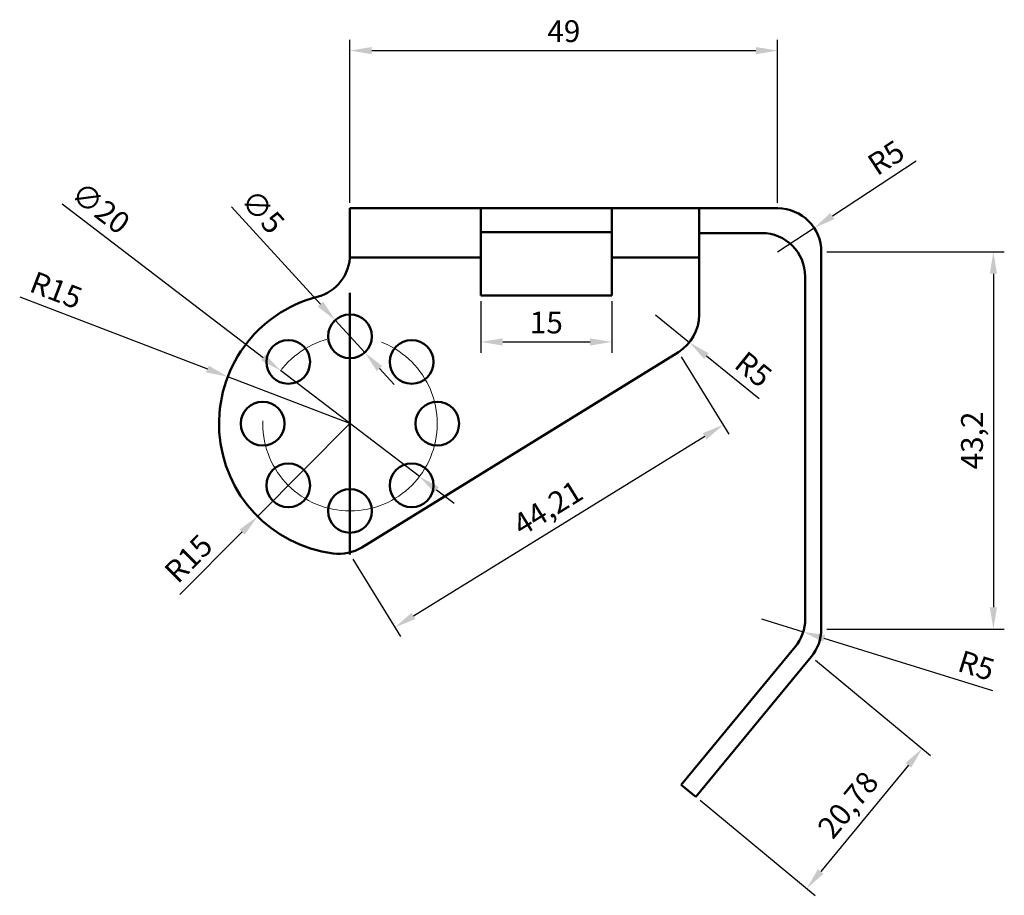
# Model space of a CAD drawing. Units: millimetres. Extents: x 1154 to 1562, y 1225 to 1481.
# Tile 4 of 4: x 1395 to 1508, y 1374 to 1475. Entities that reach past the tile are written whole.
import ezdxf

# ---------------------------------------------------------------- set-up
doc = ezdxf.new("R2010")
doc.units = ezdxf.units.MM
doc.linetypes.add('CENTER', pattern=[50.8, 31.75, -6.35, 6.35, -6.35])
for name, color, linetype, lineweight in [('M-CNTR', 1, 'CENTER', 18), ('M-DIMS', 2, 'Continuous', 25), ('M-OUTL', 7, 'Continuous', 50)]:
    doc.layers.add(name, color=color, linetype=linetype, lineweight=lineweight)
doc.styles.get("Standard").update_dxf_attribs({"font": 'arial.ttf'})
doc.dimstyles.new('ISO-25', dxfattribs={"dimtxt": 2.5, "dimasz": 2.5, "dimexe": 1.25, "dimexo": 0.625, "dimtad": 1, "dimtxsty": 'Standard', "dimcen": 2.5, "dimadec": 0, "dimazin": 0, "dimtfac": 1, "dimtmove": 0, "dimatfit": 3, "dimfxl": 1, "dimarcsym": 0})

# ---------------------------------------------------------------- blocks, each defined once
blk = doc.blocks.new('*U1')
blk.add_circle((0, 0), 2.5)
blk = doc.blocks.new('*U2')
at = {"layer": 'M-OUTL', "color": 0, "linetype": 'ByBlock', "lineweight": -2, "transparency": 16777216}
blk.add_blockref('*U1', (1432.97, 1438.42), dxfattribs=at)
for p, rotation in [((1425.9, 1435.49), 45.00000000000001), ((1440.04, 1435.49), 315), ((1422.97, 1428.42), 90), ((1442.97, 1428.42), 270), ((1425.9, 1421.35), 135), ((1440.04, 1421.35), 225), ((1432.97, 1418.42), 180)]:
    blk.add_blockref('*U1', p, dxfattribs=dict(at, rotation=rotation))
blk = doc.blocks.new('*D16')
at = {"layer": 'Defpoints', "color": 0, "transparency": 16777216}
for p in [(1481.97, 1471.15), (1432.97, 1453.09), (1481.97, 1453.09)]:
    blk.add_point(p, dxfattribs=at)
at = {"layer": 'M-DIMS', "color": 0, "lineweight": -2, "transparency": 16777216}
for p, q in [((1432.97, 1453.71), (1432.97, 1472.4)), ((1481.97, 1453.71), (1481.97, 1472.4)), ((1435.47, 1471.15), (1479.47, 1471.15))]:
    blk.add_line(p, q, dxfattribs=at)
at = {"layer": 'M-DIMS', "color": 0, "transparency": 16777216}
for points in [[(1435.47, 1471.56), (1435.47, 1470.73), (1432.97, 1471.15)], [(1479.47, 1471.56), (1479.47, 1470.73), (1481.97, 1471.15)]]:
    blk.add_solid(points, dxfattribs=at)
at = {"layer": 'M-DIMS', "color": 0, "transparency": 16777216, "insert": (1457.47, 1473.05), "char_height": 2.5, "attachment_point": 5}
blk.add_mtext('49', dxfattribs=at)
blk = doc.blocks.new('*D17')
at = {"layer": 'Defpoints', "color": 0, "transparency": 16777216}
for p in [(1486.97, 1448.09), (1486.97, 1404.89), (1506.69, 1404.89)]:
    blk.add_point(p, dxfattribs=at)
at = {"layer": 'M-DIMS', "color": 0, "lineweight": -2, "transparency": 16777216}
for p, q in [((1487.6, 1448.09), (1507.94, 1448.09)), ((1506.69, 1445.59), (1506.69, 1407.39)), ((1487.6, 1404.89), (1507.94, 1404.89))]:
    blk.add_line(p, q, dxfattribs=at)
at = {"layer": 'M-DIMS', "color": 0, "transparency": 16777216}
for points in [[(1506.27, 1445.59), (1507.1, 1445.59), (1506.69, 1448.09)], [(1506.27, 1407.39), (1507.1, 1407.39), (1506.69, 1404.89)]]:
    blk.add_solid(points, dxfattribs=at)
at = {"layer": 'M-DIMS', "color": 0, "transparency": 16777216, "insert": (1504.56, 1426.49), "char_height": 2.5, "attachment_point": 5, "rotation": 90}
blk.add_mtext('43,2', dxfattribs=at)
blk = doc.blocks.new('*D18')
at = {"layer": 'Defpoints', "color": 0, "transparency": 16777216}
for p in [(1485.83, 1401.7), (1472.6, 1385.68), (1485.31, 1375.19)]:
    blk.add_point(p, dxfattribs=at)
at = {"layer": 'M-DIMS', "color": 0, "lineweight": -2, "transparency": 16777216}
for p, q in [((1486.31, 1401.31), (1499.5, 1390.42)), ((1496.95, 1389.29), (1486.9, 1377.12)), ((1473.08, 1385.28), (1486.28, 1374.39))]:
    blk.add_line(p, q, dxfattribs=at)
at = {"layer": 'M-DIMS', "color": 0, "transparency": 16777216}
for points in [[(1496.62, 1389.55), (1497.27, 1389.02), (1498.54, 1391.22)], [(1486.58, 1377.38), (1487.22, 1376.85), (1485.31, 1375.19)]]:
    blk.add_solid(points, dxfattribs=at)
at = {"layer": 'M-DIMS', "color": 0, "transparency": 16777216, "insert": (1490.28, 1384.56), "char_height": 2.5, "attachment_point": 5, "rotation": 50.4716}
blk.add_mtext('20,78', dxfattribs=at)
blk = doc.blocks.new('*D19')
at = {"layer": 'Defpoints', "color": 0, "transparency": 16777216}
for p in [(1480.12, 1406.05), (1484.9, 1404.57)]:
    blk.add_point(p, dxfattribs=at)
at = {"layer": 'M-DIMS', "color": 0, "lineweight": -2, "transparency": 16777216}
for p, q in [((1480.12, 1406.05), (1484.9, 1404.57)), ((1506.61, 1397.81), (1487.28, 1403.82))]:
    blk.add_line(p, q, dxfattribs=at)
at = {"layer": 'M-DIMS', "color": 0, "transparency": 16777216}
blk.add_solid([(1487.41, 1404.22), (1487.16, 1403.43), (1484.9, 1404.57)], dxfattribs=at)
at = {"layer": 'M-DIMS', "color": 0, "transparency": 16777216, "insert": (1504.64, 1400.41), "char_height": 2.5, "attachment_point": 5, "rotation": 342.7219}
blk.add_mtext('R5', dxfattribs=at)
blk = doc.blocks.new('*D20')
at = {"layer": 'Defpoints', "color": 0, "transparency": 16777216}
for p in [(1486.15, 1450.83), (1481.97, 1448.09)]:
    blk.add_point(p, dxfattribs=at)
at = {"layer": 'M-DIMS', "color": 0, "lineweight": -2, "transparency": 16777216}
for p, q in [((1497.82, 1458.48), (1488.24, 1452.2)), ((1481.97, 1448.09), (1486.15, 1450.83))]:
    blk.add_line(p, q, dxfattribs=at)
at = {"layer": 'M-DIMS', "color": 0, "transparency": 16777216}
blk.add_solid([(1488.01, 1452.55), (1488.47, 1451.85), (1486.15, 1450.83)], dxfattribs=at)
at = {"layer": 'M-DIMS', "color": 0, "transparency": 16777216, "insert": (1494.56, 1458.61), "char_height": 2.5, "attachment_point": 5, "rotation": 33.2613}
blk.add_mtext('R5', dxfattribs=at)
blk = doc.blocks.new('*D21')
at = {"layer": 'Defpoints', "color": 0, "transparency": 16777216}
for p in [(1418.97, 1433.79), (1432.97, 1428.42)]:
    blk.add_point(p, dxfattribs=at)
at = {"layer": 'M-DIMS', "color": 0, "lineweight": -2, "transparency": 16777216}
for p, q in [((1395.13, 1442.93), (1416.63, 1434.68)), ((1432.97, 1428.42), (1418.97, 1433.79))]:
    blk.add_line(p, q, dxfattribs=at)
at = {"layer": 'M-DIMS', "color": 0, "transparency": 16777216}
blk.add_solid([(1416.78, 1435.07), (1416.48, 1434.29), (1418.97, 1433.79)], dxfattribs=at)
at = {"layer": 'M-DIMS', "color": 0, "transparency": 16777216, "insert": (1399.19, 1443.41), "char_height": 2.5, "attachment_point": 5, "rotation": 339.0251}
blk.add_mtext('R15', dxfattribs=at)
blk = doc.blocks.new('*D22')
at = {"layer": 'Defpoints', "color": 0, "transparency": 16777216}
for p in [(1425.02, 1434.49), (1440.92, 1422.35)]:
    blk.add_point(p, dxfattribs=at)
at = {"layer": 'M-DIMS', "color": 0, "lineweight": -2, "transparency": 16777216}
for p, q in [((1400.01, 1453.6), (1423.04, 1436.01)), ((1440.92, 1422.35), (1425.02, 1434.49)), ((1442.9, 1420.83), (1444.89, 1419.31))]:
    blk.add_line(p, q, dxfattribs=at)
at = {"layer": 'M-DIMS', "color": 0, "transparency": 16777216}
for points in [[(1423.29, 1436.34), (1422.79, 1435.68), (1425.02, 1434.49)], [(1443.16, 1421.16), (1442.65, 1420.5), (1440.92, 1422.35)]]:
    blk.add_solid(points, dxfattribs=at)
at = {"layer": 'M-DIMS', "color": 0, "transparency": 16777216, "insert": (1404.21, 1452.87), "char_height": 2.5, "attachment_point": 5, "rotation": 322.6228}
blk.add_mtext('∅20', dxfattribs=at)
blk = doc.blocks.new('*D23')
at = {"layer": 'Defpoints', "color": 0, "transparency": 16777216}
for p in [(1431.28, 1440.26), (1434.66, 1436.58)]:
    blk.add_point(p, dxfattribs=at)
at = {"layer": 'M-DIMS', "color": 0, "lineweight": -2, "transparency": 16777216}
for p, q in [((1419.39, 1453.25), (1429.59, 1442.11)), ((1434.66, 1436.58), (1431.28, 1440.26)), ((1436.35, 1434.73), (1438.04, 1432.89))]:
    blk.add_line(p, q, dxfattribs=at)
at = {"layer": 'M-DIMS', "color": 0, "transparency": 16777216}
for points in [[(1429.9, 1442.39), (1429.29, 1441.82), (1431.28, 1440.26)], [(1436.66, 1435.01), (1436.04, 1434.45), (1434.66, 1436.58)]]:
    blk.add_solid(points, dxfattribs=at)
at = {"layer": 'M-DIMS', "color": 0, "transparency": 16777216, "insert": (1422.74, 1452.5), "char_height": 2.5, "attachment_point": 5, "rotation": 312.4942}
blk.add_mtext('∅5', dxfattribs=at)
blk = doc.blocks.new('*D24')
at = {"layer": 'Defpoints', "color": 0, "transparency": 16777216}
for p in [(1467.97, 1440.88), (1471.86, 1437.73)]:
    blk.add_point(p, dxfattribs=at)
at = {"layer": 'M-DIMS', "color": 0, "lineweight": -2, "transparency": 16777216}
for p, q in [((1467.97, 1440.88), (1471.86, 1437.73)), ((1479.86, 1431.25), (1473.8, 1436.16))]:
    blk.add_line(p, q, dxfattribs=at)
at = {"layer": 'M-DIMS', "color": 0, "transparency": 16777216}
blk.add_solid([(1474.06, 1436.48), (1473.54, 1435.83), (1471.86, 1437.73)], dxfattribs=at)
at = {"layer": 'M-DIMS', "color": 0, "transparency": 16777216, "insert": (1478.99, 1434.39), "char_height": 2.5, "attachment_point": 5, "rotation": 320.9715}
blk.add_mtext('R5', dxfattribs=at)
blk = doc.blocks.new('*D25')
at = {"layer": 'Defpoints', "color": 0, "transparency": 16777216}
for p in [(1447.97, 1443.09), (1462.97, 1443.09), (1462.97, 1437.78)]:
    blk.add_point(p, dxfattribs=at)
at = {"layer": 'M-DIMS', "color": 0, "lineweight": -2, "transparency": 16777216}
for p, q in [((1447.97, 1442.46), (1447.97, 1436.53)), ((1462.97, 1442.46), (1462.97, 1436.53)), ((1450.47, 1437.78), (1460.47, 1437.78))]:
    blk.add_line(p, q, dxfattribs=at)
at = {"layer": 'M-DIMS', "color": 0, "transparency": 16777216}
for points in [[(1450.47, 1438.19), (1450.47, 1437.36), (1447.97, 1437.78)], [(1460.47, 1438.19), (1460.47, 1437.36), (1462.97, 1437.78)]]:
    blk.add_solid(points, dxfattribs=at)
at = {"layer": 'M-DIMS', "color": 0, "transparency": 16777216, "insert": (1455.47, 1439.68), "char_height": 2.5, "attachment_point": 5}
blk.add_mtext('15', dxfattribs=at)
blk = doc.blocks.new('*D58')
at = {"layer": 'Defpoints', "color": 0, "transparency": 16777216}
for p in [(1470.6, 1436.62), (1475.74, 1428.29), (1432.97, 1413.42)]:
    blk.add_point(p, dxfattribs=at)
at = {"layer": 'M-DIMS', "color": 0, "lineweight": -2, "transparency": 16777216}
for p, q in [((1470.92, 1436.09), (1476.39, 1427.22)), ((1440.24, 1406.39), (1473.61, 1426.97)), ((1433.3, 1412.89), (1438.77, 1404.02))]:
    blk.add_line(p, q, dxfattribs=at)
at = {"layer": 'M-DIMS', "color": 0, "transparency": 16777216}
for points in [[(1473.39, 1427.33), (1473.83, 1426.62), (1475.74, 1428.29)], [(1440.02, 1406.75), (1440.46, 1406.04), (1438.11, 1405.08)]]:
    blk.add_solid(points, dxfattribs=at)
at = {"layer": 'M-DIMS', "color": 0, "transparency": 16777216, "insert": (1455.81, 1418.49), "char_height": 2.5, "attachment_point": 5, "rotation": 31.6642}
blk.add_mtext('44,21', dxfattribs=at)
blk = doc.blocks.new('*D99')
at = {"layer": 'Defpoints', "color": 0, "transparency": 16777216}
for p in [(1432.97, 1428.42), (1422.39, 1417.79)]:
    blk.add_point(p, dxfattribs=at)
at = {"layer": 'M-DIMS', "color": 0, "lineweight": -2, "transparency": 16777216}
for p, q in [((1432.97, 1428.42), (1422.39, 1417.79)), ((1413.48, 1408.84), (1420.63, 1416.02))]:
    blk.add_line(p, q, dxfattribs=at)
at = {"layer": 'M-DIMS', "color": 0, "transparency": 16777216}
blk.add_solid([(1420.33, 1416.31), (1420.92, 1415.72), (1422.39, 1417.79)], dxfattribs=at)
at = {"layer": 'M-DIMS', "color": 0, "transparency": 16777216, "insert": (1414.69, 1412.75), "char_height": 2.5, "attachment_point": 5, "rotation": 45.1309}
blk.add_mtext('R15', dxfattribs=at)

msp = doc.modelspace()

# ---------------------------------------------------------------- linework, layer by layer
at = {"layer": 'M-CNTR'}
msp.add_circle((1432.9713, 1428.4197), 10, dxfattribs=at)
at = {"layer": 'M-OUTL'}
for p, q in [((1432.9713, 1447.7846), (1432.9713, 1453.0897)), ((1432.9713, 1453.0897), (1481.9713, 1453.0897)), ((1432.9713, 1453.0897), (1472.9713, 1453.0897)), ((1447.9713, 1443.0897), (1447.9713, 1453.0897)), ((1472.9713, 1453.0897), (1462.9713, 1453.0897)), ((1462.9713, 1453.0897), (1462.9713, 1443.0897)), ((1472.9713, 1453.0897), (1472.9713, 1440.8804)), ((1447.9713, 1450.3494), (1462.9713, 1450.3494)), ((1472.9713, 1450.2565), (1480.1228, 1450.2565)), ((1432.9713, 1447.4683), (1447.9713, 1447.4683)), ((1462.9713, 1447.4683), (1472.9713, 1447.4683)), ((1486.9713, 1448.0897), (1486.9713, 1404.8863)), ((1485.1228, 1445.2565), (1485.1228, 1406.0517)), ((1432.9713, 1443.4197), (1432.9713, 1413.4197)), ((1462.9713, 1443.0897), (1447.9713, 1443.0897)), ((1470.596, 1436.6247), (1434.3122, 1414.2467)), ((1483.9793, 1402.8694), (1470.9305, 1387.0559)), ((1485.8278, 1401.704), (1472.6024, 1385.6764)), ((1470.9305, 1387.0559), (1472.6024, 1385.6764))]:
    msp.add_line(p, q, dxfattribs=at)
for centre, radius, start, end in [((1481.9713, 1448.0897), 5, 0, 90), ((1480.1228, 1445.2565), 5, 0, 90), ((1427.9713, 1447.7846), 5, 284.477512, 0), ((1432.9713, 1428.4197), 15, 104.477512, 262.624424), ((1467.9713, 1440.8804), 5, 301.66421, 0), ((1431.6875, 1418.5024), 5, 262.624424, 301.66421), ((1480.1228, 1406.0517), 5, 320.471604, 0), ((1481.9713, 1404.8863), 5, 320.471604, 0)]:
    msp.add_arc(centre, radius, start, end, dxfattribs=at)

# ---------------------------------------------------------------- block references
msp.add_blockref('*U2', (0, 0), dxfattribs=at)

# ---------------------------------------------------------------- dimensions: what is measured, and where the dimension line sits
at = {"layer": 'M-DIMS'}
for base, p1, p2, picture, middle in [((1481.9713, 1471.1474), (1432.9713, 1453.0897), (1481.9713, 1453.0897), '*D16', (1457.4713, 1473.0489)), ((1462.9713, 1437.7753), (1447.9713, 1443.0897), (1462.9713, 1443.0897), '*D25', (1455.4713, 1439.6767))]:
    dim = msp.add_linear_dim(base=base, p1=p1, p2=p2, dimstyle='ISO-25', override={"dimclrd": 0, "dimclre": 0, "dimclrt": 0}, dxfattribs=at)
    dim.commit()
    dim.dimension.update_dxf_attribs({"geometry": picture, "text_midpoint": middle})
for center, mpoint, override, picture, middle in [((1481.9713, 1448.0897), (1486.1522, 1450.832), {"dimclrd": 0, "dimclre": 0, "dimclrt": 0}, '*D20', (1495.6001, 1457.029)), ((1432.9713, 1428.4197), (1418.9652, 1433.7891), {"dimclrd": 0, "dimclre": 0, "dimclrt": 0}, '*D21', (1398.5094, 1441.631)), ((1432.9713, 1428.4197), (1422.3889, 1417.7889), {"dimdec": 0, "dimlfac": 1, "dimrnd": 0, "dimzin": 0, "dimdsep": 46, "dimlunit": 2}, '*D99', (1416.0395, 1411.4104)), ((1480.1228, 1406.0517), (1484.8971, 1404.5667), {"dimclrd": 0, "dimclre": 0, "dimclrt": 0}, '*D19', (1504.0786, 1398.6004))]:
    dim = msp.add_radius_dim(center=center, mpoint=mpoint, dimstyle='ISO-25', override=override, dxfattribs=at)
    dim.commit()
    dim.dimension.update_dxf_attribs({"geometry": picture, "text_midpoint": middle, "dimtype": 164})
for p1, p2, picture, middle in [((1440.9178, 1422.3491), (1425.0247, 1434.4903), '*D22', (1403.0107, 1451.3074)), ((1434.6601, 1436.5763), (1431.2825, 1440.263), '*D23', (1421.2891, 1451.1711))]:
    dim = msp.add_diameter_dim_2p(p1=p1, p2=p2, dimstyle='ISO-25', override={"dimclrd": 0, "dimclre": 0, "dimclrt": 0}, dxfattribs=at)
    dim.commit()
    dim.dimension.update_dxf_attribs({"geometry": picture, "text_midpoint": middle, "dimtype": 163})
dim = msp.add_linear_dim(base=(1506.6873, 1404.8863), p1=(1486.9713, 1448.0897), p2=(1486.9713, 1404.8863), angle=90, dimstyle='ISO-25', override={"dimclrd": 0, "dimclre": 0, "dimclrt": 0}, dxfattribs=at)
dim.commit()
dim.dimension.update_dxf_attribs({"geometry": '*D17', "text_midpoint": (1504.5599, 1426.488)})
dim = msp.add_radius_dim(center=(1467.9713, 1440.8804), mpoint=(1471.8554, 1437.7319), dimstyle='ISO-25', override={"dimclrd": 0, "dimclre": 0, "dimclrt": 0}, dxfattribs=at)
dim.commit()
dim.dimension.update_dxf_attribs({"geometry": '*D24', "text_midpoint": (1478.9924, 1434.3877)})
for p1, p2, distance, picture, middle in [((1432.9713, 1413.4197), (1470.596, 1436.6247), -9.7962, '*D58', (1455.8093, 1418.4949)), ((1485.8278, 1401.704), (1472.6024, 1385.6764), 16.4775, '*D18', (1490.2835, 1384.5569))]:
    dim = msp.add_aligned_dim(p1=p1, p2=p2, distance=distance, dimstyle='ISO-25', override={"dimclrd": 0, "dimclre": 0, "dimclrt": 0}, dxfattribs=at)
    dim.commit()
    dim.dimension.update_dxf_attribs({"geometry": picture, "text_midpoint": middle})

doc.saveas('drawing.dxf')
